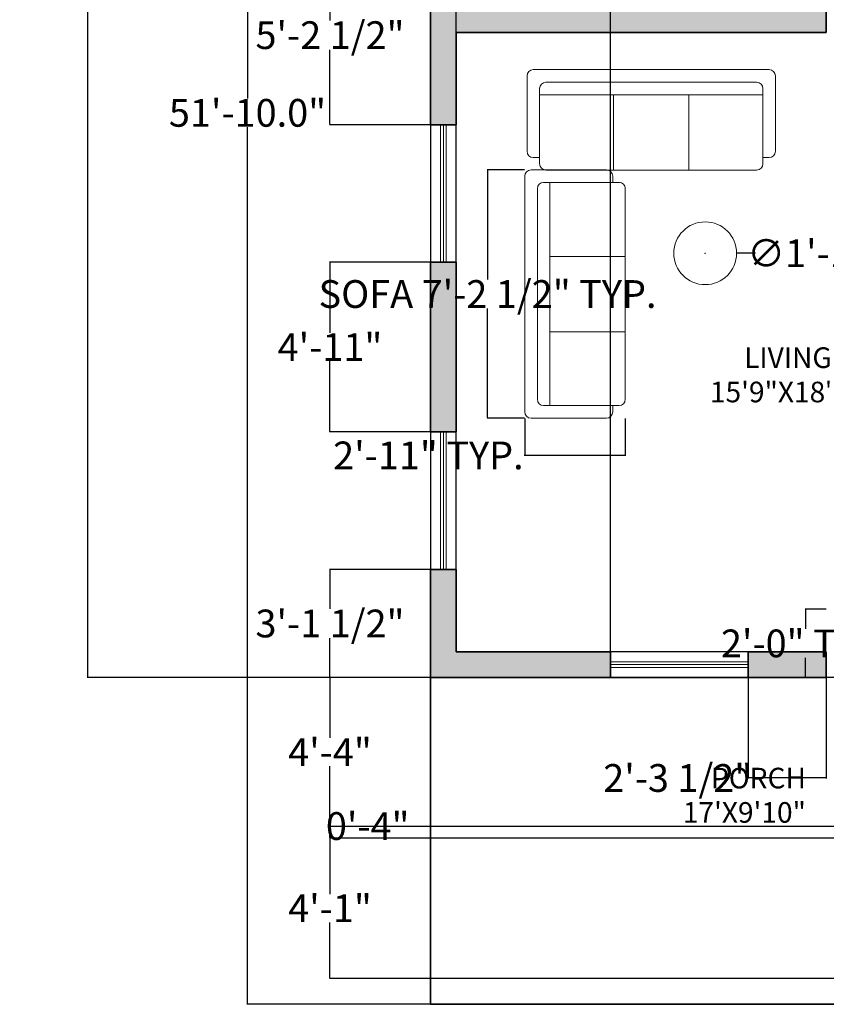
# Model space of a CAD drawing. Units: inches. Extents: x 2103 to 2702, y 2405 to 3142.
# Tile 1 of 7: x 2103 to 2384, y 2447 to 2790. Entities that reach past the tile are written whole.
import ezdxf

# ---------------------------------------------------------------- set-up
doc = ezdxf.new("R2010")
doc.units = ezdxf.units.IN
doc.linetypes.add('0', pattern=[0])
for name, color, linetype, lineweight in [('00 FURNITURE', 15, 'Continuous', 15), ('A-ANNO-DIMS', 2, 'Continuous', 18), ('A-AREA-IDEN', 7, 'Continuous', 18), ('A-WALL-PATT', 8, 'Continuous', 9), ('WALL', 7, 'Continuous', 35), ('WINDOW', 160, '0', 5), ('windows', 4, 'Continuous', 18)]:
    doc.layers.add(name, color=color, linetype=linetype, lineweight=lineweight)
doc.layers.add('furniture', color=34, linetype='Continuous')
doc.styles.get("Standard").update_dxf_attribs({"font": 'arial.ttf'})
doc.dimstyles.get("Standard").update_dxf_attribs({"dimtxt": 9.68, "dimasz": 0.18, "dimexe": 0.18, "dimexo": 0.0625, "dimgap": 0.09, "dimtad": 0, "dimtih": 1, "dimtoh": 1, "dimdec": 1, "dimzin": 0, "dimdsep": 46, "dimlunit": 3, "dimtxsty": 'Standard', "dimcen": 0.09, "dimadec": 0, "dimazin": 0, "dimtfac": 1, "dimtdec": 1, "dimtofl": 0, "dimtmove": 0, "dimatfit": 3, "dimfxl": 1, "dimtolj": 1, "dimtzin": 0, "dimarcsym": 0})

# ---------------------------------------------------------------- blocks, each defined once
blk = doc.blocks.new('window')
at = {"layer": 'furniture'}
for p, q in [((1745.13, 2764.08), (1745.13, 2716.08)), ((1754.13, 2716.08), (1754.13, 2764.08))]:
    blk.add_line(p, q, dxfattribs=at)
at = {"layer": 'WINDOW'}
for p, q in [((1748.63, 2764.08), (1748.63, 2716.08)), ((1749.63, 2764.08), (1749.63, 2716.08)), ((1750.63, 2764.08), (1750.63, 2716.08))]:
    blk.add_line(p, q, dxfattribs=at)
blk = doc.blocks.new('sofa 6')
for p, q in [((-1044.4, 890), (1044.4, 890)), ((-1100, 166.9), (-1100, 834.3)), ((1100, 834.3), (1100, 166.9)), ((-988.8, 55.6), (-988.8, 723.1)), ((-933.1, 778.7), (933.1, 778.7)), ((988.8, 723.1), (988.8, 55.6)), ((-988.8, 667.5), (988.8, 667.5)), ((-333.8, 667.5), (-333.8, 0)), ((333.7, 667.5), (333.7, 0)), ((-988.8, 111.2), (-1044.4, 111.2)), ((1044.4, 111.2), (988.8, 111.2)), ((933.1, 0), (-933.1, 0))]:
    blk.add_line(p, q)
for centre, start, end in [((-1044.4, 834.3), 90, 180), ((1044.4, 834.3), 0, 90), ((-933.1, 723.1), 90, 180), ((933.1, 723.1), 0, 90), ((-1044.4, 166.9), 180, 270), ((1044.4, 166.9), 270, 0), ((-933.1, 55.6), 180, 270), ((933.1, 55.6), 270, 0)]:
    blk.add_arc(centre, 55.6, start, end)
blk = doc.blocks.new('*D16')
at = {"layer": 'A-ANNO-DIMS', "color": 0, "lineweight": -2, "transparency": 16777216}
for p, q in [((2246.37, 3068.85), (2182.44, 3068.85)), ((2182.62, 3068.67), (2182.62, 2762.88)), ((2182.62, 2447.03), (2182.62, 2752.81)), ((2246.37, 2446.85), (2182.44, 2446.85))]:
    blk.add_line(p, q, dxfattribs=at)
at = {"layer": 'A-ANNO-DIMS', "color": 0, "transparency": 16777216}
for points in [[(2182.59, 3068.67), (2182.65, 3068.67), (2182.62, 3068.85)], [(2182.59, 2447.03), (2182.65, 2447.03), (2182.62, 2446.85)]]:
    blk.add_solid(points, dxfattribs=at)
at = {"layer": 'Defpoints', "color": 0, "transparency": 16777216}
for p in [(2246.43, 3068.85), (2182.62, 2446.85), (2246.43, 2446.85)]:
    blk.add_point(p, dxfattribs=at)
at = {"layer": 'A-ANNO-DIMS', "color": 0, "transparency": 16777216, "insert": (2182.62, 2757.85), "char_height": 9.68, "attachment_point": 5}
blk.add_mtext('\\A1;51\'-10.0"', dxfattribs=at)
blk = doc.blocks.new('*D17')
at = {"layer": 'A-ANNO-DIMS', "color": 0, "lineweight": -2, "transparency": 16777216}
for p, q in [((2246.37, 3068.85), (2126.76, 3068.85)), ((2126.94, 3068.67), (2126.94, 2819.88)), ((2126.94, 2561.03), (2126.94, 2809.81)), ((2246.37, 2560.85), (2126.76, 2560.85))]:
    blk.add_line(p, q, dxfattribs=at)
at = {"layer": 'A-ANNO-DIMS', "color": 0, "transparency": 16777216}
for points in [[(2126.91, 3068.67), (2126.97, 3068.67), (2126.94, 3068.85)], [(2126.91, 2561.03), (2126.97, 2561.03), (2126.94, 2560.85)]]:
    blk.add_solid(points, dxfattribs=at)
at = {"layer": 'Defpoints', "color": 0, "transparency": 16777216}
for p in [(2246.43, 3068.85), (2126.94, 2560.85), (2246.43, 2560.85)]:
    blk.add_point(p, dxfattribs=at)
at = {"layer": 'A-ANNO-DIMS', "color": 0, "transparency": 16777216, "insert": (2126.94, 2814.85), "char_height": 9.68, "attachment_point": 5}
blk.add_mtext('\\A1;42\'-4.0"', dxfattribs=at)
blk = doc.blocks.new('*D27')
at = {"layer": 'A-ANNO-DIMS', "color": 0, "lineweight": -2, "transparency": 16777216}
for p, q in [((2384.37, 2584.67), (2377.05, 2584.67)), ((2377.23, 2584.49), (2377.23, 2577.79)), ((2377.23, 2561.03), (2377.23, 2567.72)), ((2384.37, 2560.85), (2377.05, 2560.85))]:
    blk.add_line(p, q, dxfattribs=at)
at = {"layer": 'A-ANNO-DIMS', "color": 0, "transparency": 16777216}
for points in [[(2377.2, 2584.49), (2377.26, 2584.49), (2377.23, 2584.67)], [(2377.2, 2561.03), (2377.26, 2561.03), (2377.23, 2560.85)]]:
    blk.add_solid(points, dxfattribs=at)
at = {"layer": 'Defpoints', "color": 0, "transparency": 16777216}
for p in [(2384.43, 2584.67), (2377.23, 2560.85), (2384.43, 2560.85)]:
    blk.add_point(p, dxfattribs=at)
at = {"layer": 'A-ANNO-DIMS', "color": 0, "transparency": 16777216, "insert": (2377.23, 2572.76), "char_height": 9.68, "attachment_point": 5}
blk.add_mtext('\\A1;2\'-0" TYP.', dxfattribs=at)
blk = doc.blocks.new('*D30')
at = {"layer": 'A-ANNO-DIMS', "color": 0, "lineweight": -2, "transparency": 16777216}
for p, q in [((2279.24, 2737.95), (2266.13, 2737.95)), ((2266.31, 2737.77), (2266.31, 2699.74)), ((2266.31, 2651.51), (2266.31, 2689.54)), ((2279.24, 2651.33), (2266.13, 2651.33))]:
    blk.add_line(p, q, dxfattribs=at)
at = {"layer": 'A-ANNO-DIMS', "color": 0, "transparency": 16777216}
for points in [[(2266.28, 2737.77), (2266.34, 2737.77), (2266.31, 2737.95)], [(2266.28, 2651.51), (2266.34, 2651.51), (2266.31, 2651.33)]]:
    blk.add_solid(points, dxfattribs=at)
at = {"layer": 'Defpoints', "color": 0, "transparency": 16777216}
for p in [(2266.31, 2737.95), (2279.31, 2737.95), (2279.31, 2651.33)]:
    blk.add_point(p, dxfattribs=at)
at = {"layer": 'A-ANNO-DIMS', "color": 0, "transparency": 16777216, "insert": (2266.31, 2694.64), "char_height": 9.68, "attachment_point": 5}
blk.add_mtext('\\A1;SOFA 7\'-2 1/2" TYP.', dxfattribs=at)
blk = doc.blocks.new('*D31')
at = {"layer": 'A-ANNO-DIMS', "color": 0, "lineweight": -2, "transparency": 16777216}
for p, q in [((2279.31, 2651.27), (2279.31, 2638.16)), ((2314.34, 2651.27), (2314.34, 2638.16)), ((2279.31, 2638.34), (2279.13, 2638.34)), ((2314.16, 2638.34), (2279.49, 2638.34))]:
    blk.add_line(p, q, dxfattribs=at)
at = {"layer": 'A-ANNO-DIMS', "color": 0, "transparency": 16777216}
for points in [[(2279.49, 2638.37), (2279.49, 2638.31), (2279.31, 2638.34)], [(2314.16, 2638.37), (2314.16, 2638.31), (2314.34, 2638.34)]]:
    blk.add_solid(points, dxfattribs=at)
at = {"layer": 'Defpoints', "color": 0, "transparency": 16777216}
for p in [(2279.31, 2651.33), (2314.34, 2651.33), (2279.31, 2638.34)]:
    blk.add_point(p, dxfattribs=at)
at = {"layer": 'A-ANNO-DIMS', "color": 0, "transparency": 16777216, "insert": (2245.69, 2638.34), "char_height": 9.68, "attachment_point": 5}
blk.add_mtext('\\A1;2\'-11" TYP.', dxfattribs=at)
blk = doc.blocks.new('*D42')
at = {"layer": 'A-ANNO-DIMS', "color": 0, "lineweight": -2, "transparency": 16777216}
for p, q in [((2471.37, 2504.85), (2211.2, 2504.85)), ((2211.38, 2504.67), (2211.38, 2485.3)), ((2211.38, 2456.03), (2211.38, 2475.4)), ((2471.37, 2455.85), (2211.2, 2455.85))]:
    blk.add_line(p, q, dxfattribs=at)
at = {"layer": 'A-ANNO-DIMS', "color": 0, "transparency": 16777216}
for points in [[(2211.35, 2504.67), (2211.41, 2504.67), (2211.38, 2504.85)], [(2211.35, 2456.03), (2211.41, 2456.03), (2211.38, 2455.85)]]:
    blk.add_solid(points, dxfattribs=at)
at = {"layer": 'Defpoints', "color": 0, "transparency": 16777216}
for p in [(2211.38, 2504.85), (2471.43, 2504.85), (2471.43, 2455.85)]:
    blk.add_point(p, dxfattribs=at)
at = {"layer": 'A-ANNO-DIMS', "color": 0, "transparency": 16777216, "insert": (2211.38, 2480.35), "char_height": 9.68, "attachment_point": 5}
blk.add_mtext('\\A1;4\'-1"', dxfattribs=at)
blk = doc.blocks.new('*D43')
at = {"layer": 'A-ANNO-DIMS', "color": 0, "lineweight": -2, "transparency": 16777216}
for p, q in [((2471.367635, 2560.845674), (2211.200134, 2560.845674)), ((2211.380134, 2560.665674), (2211.380134, 2539.775674)), ((2211.380134, 2509.025674), (2211.380134, 2529.915674)), ((2471.367635, 2508.845674), (2211.200134, 2508.845674))]:
    blk.add_line(p, q, dxfattribs=at)
at = {"layer": 'A-ANNO-DIMS', "color": 0, "transparency": 16777216}
for points in [[(2211.350134, 2560.665674), (2211.410134, 2560.665674), (2211.380134, 2560.845674)], [(2211.350134, 2509.025674), (2211.410134, 2509.025674), (2211.380134, 2508.845674)]]:
    blk.add_solid(points, dxfattribs=at)
at = {"layer": 'Defpoints', "color": 0, "transparency": 16777216}
for p in [(2211.380134, 2560.845674), (2471.430135, 2560.845674), (2471.430135, 2508.845674)]:
    blk.add_point(p, dxfattribs=at)
at = {"layer": 'A-ANNO-DIMS', "color": 0, "transparency": 16777216, "insert": (2211.380134, 2534.845674), "char_height": 9.68, "attachment_point": 5}
blk.add_mtext('\\A1;4\'-4"', dxfattribs=at)
blk = doc.blocks.new('*D47')
at = {"layer": 'A-ANNO-DIMS', "color": 0, "lineweight": -2, "transparency": 16777216}
for p, q in [((2471.37, 2508.85), (2211.2, 2508.85)), ((2211.38, 2508.85), (2211.38, 2509.03)), ((2211.38, 2509.03), (2211.56, 2509.03)), ((2211.38, 2505.03), (2211.38, 2508.67)), ((2471.37, 2504.85), (2211.2, 2504.85))]:
    blk.add_line(p, q, dxfattribs=at)
at = {"layer": 'A-ANNO-DIMS', "color": 0, "transparency": 16777216}
for points in [[(2211.35, 2508.67), (2211.41, 2508.67), (2211.38, 2508.85)], [(2211.35, 2505.03), (2211.41, 2505.03), (2211.38, 2504.85)]]:
    blk.add_solid(points, dxfattribs=at)
at = {"layer": 'Defpoints', "color": 0, "transparency": 16777216}
for p in [(2211.38, 2508.85), (2471.43, 2508.85), (2471.43, 2504.85)]:
    blk.add_point(p, dxfattribs=at)
at = {"layer": 'A-ANNO-DIMS', "color": 0, "transparency": 16777216, "insert": (2224.52, 2509.03), "char_height": 9.68, "attachment_point": 5}
blk.add_mtext('\\A1;0\'-4"', dxfattribs=at)
blk = doc.blocks.new('*D48')
at = {"layer": 'A-ANNO-DIMS', "color": 0, "lineweight": -2, "transparency": 16777216}
for p, q in [((2255.43, 2569.91), (2255.43, 3118.9)), ((2255.61, 3118.72), (2257.85, 3118.72)), ((2308.95, 3118.72), (2306.71, 3118.72)), ((2309.13, 2569.91), (2309.13, 3118.9))]:
    blk.add_line(p, q, dxfattribs=at)
at = {"layer": 'A-ANNO-DIMS', "color": 0, "transparency": 16777216}
for points in [[(2255.61, 3118.75), (2255.61, 3118.69), (2255.43, 3118.72)], [(2308.95, 3118.75), (2308.95, 3118.69), (2309.13, 3118.72)]]:
    blk.add_solid(points, dxfattribs=at)
at = {"layer": 'Defpoints', "color": 0, "transparency": 16777216}
for p in [(2309.13, 3118.72), (2255.43, 2569.85), (2309.13, 2569.85)]:
    blk.add_point(p, dxfattribs=at)
at = {"layer": 'A-ANNO-DIMS', "color": 0, "transparency": 16777216, "insert": (2282.28, 3118.72), "char_height": 9.68, "attachment_point": 5}
blk.add_mtext('\\A1;4\'-5 1/2"', dxfattribs=at)
blk = doc.blocks.new('*D49')
at = {"layer": 'A-ANNO-DIMS', "color": 0, "lineweight": -2, "transparency": 16777216}
for p, q in [((2357.13, 2560.78), (2357.13, 2525.62)), ((2384.43, 2560.78), (2384.43, 2525.62)), ((2357.13, 2525.8), (2356.95, 2525.8)), ((2384.25, 2525.8), (2357.31, 2525.8))]:
    blk.add_line(p, q, dxfattribs=at)
at = {"layer": 'A-ANNO-DIMS', "color": 0, "transparency": 16777216}
for points in [[(2357.31, 2525.83), (2357.31, 2525.77), (2357.13, 2525.8)], [(2384.25, 2525.83), (2384.25, 2525.77), (2384.43, 2525.8)]]:
    blk.add_solid(points, dxfattribs=at)
at = {"layer": 'Defpoints', "color": 0, "transparency": 16777216}
for p in [(2357.13, 2560.85), (2384.43, 2560.85), (2357.13, 2525.8)]:
    blk.add_point(p, dxfattribs=at)
at = {"layer": 'A-ANNO-DIMS', "color": 0, "transparency": 16777216, "insert": (2332.63, 2525.8), "char_height": 9.68, "attachment_point": 5}
blk.add_mtext('\\A1;2\'-3 1/2"', dxfattribs=at)
blk = doc.blocks.new('*D51')
at = {"layer": 'A-ANNO-DIMS', "color": 0, "lineweight": -2, "transparency": 16777216}
for p, q in [((2246.37, 2598.55), (2211.2, 2598.55)), ((2211.38, 2598.37), (2211.38, 2584.8)), ((2211.38, 2561.03), (2211.38, 2574.6)), ((2246.37, 2560.85), (2211.2, 2560.85))]:
    blk.add_line(p, q, dxfattribs=at)
at = {"layer": 'A-ANNO-DIMS', "color": 0, "transparency": 16777216}
for points in [[(2211.35, 2598.37), (2211.41, 2598.37), (2211.38, 2598.55)], [(2211.35, 2561.03), (2211.41, 2561.03), (2211.38, 2560.85)]]:
    blk.add_solid(points, dxfattribs=at)
at = {"layer": 'Defpoints', "color": 0, "transparency": 16777216}
for p in [(2211.38, 2598.55), (2246.43, 2598.55), (2246.43, 2560.85)]:
    blk.add_point(p, dxfattribs=at)
at = {"layer": 'A-ANNO-DIMS', "color": 0, "transparency": 16777216, "insert": (2211.38, 2579.7), "char_height": 9.68, "attachment_point": 5}
blk.add_mtext('\\A1;3\'-1 1/2"', dxfattribs=at)
blk = doc.blocks.new('*D52')
at = {"layer": 'A-ANNO-DIMS', "color": 0, "lineweight": -2, "transparency": 16777216}
for p, q in [((2246.37, 2705.7), (2211.2, 2705.7)), ((2211.38, 2705.52), (2211.38, 2681.08)), ((2211.38, 2646.73), (2211.38, 2671.18)), ((2246.37, 2646.55), (2211.2, 2646.55))]:
    blk.add_line(p, q, dxfattribs=at)
at = {"layer": 'A-ANNO-DIMS', "color": 0, "transparency": 16777216}
for points in [[(2211.35, 2705.52), (2211.41, 2705.52), (2211.38, 2705.7)], [(2211.35, 2646.73), (2211.41, 2646.73), (2211.38, 2646.55)]]:
    blk.add_solid(points, dxfattribs=at)
at = {"layer": 'Defpoints', "color": 0, "transparency": 16777216}
for p in [(2211.38, 2705.7), (2246.43, 2705.7), (2246.43, 2646.55)]:
    blk.add_point(p, dxfattribs=at)
at = {"layer": 'A-ANNO-DIMS', "color": 0, "transparency": 16777216, "insert": (2211.38, 2676.13), "char_height": 9.68, "attachment_point": 5}
blk.add_mtext('\\A1;4\'-11"', dxfattribs=at)
blk = doc.blocks.new('*D53')
at = {"layer": 'A-ANNO-DIMS', "color": 0, "lineweight": -2, "transparency": 16777216}
for p, q in [((2246.37, 2816.19), (2211.2, 2816.19)), ((2211.38, 2816.01), (2211.38, 2790.04)), ((2211.38, 2753.88), (2211.38, 2779.85)), ((2246.37, 2753.7), (2211.2, 2753.7))]:
    blk.add_line(p, q, dxfattribs=at)
at = {"layer": 'A-ANNO-DIMS', "color": 0, "transparency": 16777216}
for points in [[(2211.35, 2816.01), (2211.41, 2816.01), (2211.38, 2816.19)], [(2211.35, 2753.88), (2211.41, 2753.88), (2211.38, 2753.7)]]:
    blk.add_solid(points, dxfattribs=at)
at = {"layer": 'Defpoints', "color": 0, "transparency": 16777216}
for p in [(2211.38, 2816.19), (2246.43, 2816.19), (2246.43, 2753.7)]:
    blk.add_point(p, dxfattribs=at)
at = {"layer": 'A-ANNO-DIMS', "color": 0, "transparency": 16777216, "insert": (2211.38, 2784.95), "char_height": 9.68, "attachment_point": 5}
blk.add_mtext('\\A1;5\'-2 1/2"', dxfattribs=at)
blk = doc.blocks.new('*D78')
at = {"layer": 'A-ANNO-DIMS', "color": 0, "lineweight": -2, "transparency": 16777216}
for p, q in [((2342.12, 2708.86), (2342.3, 2708.86)), ((2342.21, 2708.77), (2342.21, 2708.95)), ((2359.73, 2708.87), (2353.34, 2708.86))]:
    blk.add_line(p, q, dxfattribs=at)
at = {"layer": 'A-ANNO-DIMS', "color": 0, "transparency": 16777216}
blk.add_solid([(2353.34, 2708.9), (2353.34, 2708.84), (2353.16, 2708.86)], dxfattribs=at)
at = {"layer": 'Defpoints', "color": 0, "transparency": 16777216}
for p in [(2331.26, 2708.86), (2353.16, 2708.86)]:
    blk.add_point(p, dxfattribs=at)
at = {"layer": 'A-ANNO-DIMS', "color": 0, "transparency": 16777216, "insert": (2381.71, 2708.87), "char_height": 9.68, "attachment_point": 5}
blk.add_mtext('\\A1;∅1\'-10"', dxfattribs=at)

msp = doc.modelspace()

# ---------------------------------------------------------------- hatches: boundary and pattern name
at = {"layer": 'A-WALL-PATT'}
h = msp.add_hatch(color=256, dxfattribs=at)
h.dxf.hatch_style = 1
h.paths.add_polyline_path([(2342.43, 2911.85), (2342.43, 2915.85), (2255.43, 2915.85), (2255.43, 2976.23), (2246.43, 2976.23), (2246.43, 2840.19), (2255.43, 2840.19), (2255.43, 2854.85), (2315.43, 2854.85), (2315.43, 2845.85), (2319.43, 2845.85), (2319.43, 2858.85), (2255.43, 2858.85), (2255.43, 2906.85), (2342.43, 2906.85)])
h.paths.add_polyline_path([(2384.43, 2794.85), (2319.43, 2794.85), (2319.43, 2815.85), (2315.43, 2815.85), (2315.43, 2794.85), (2255.43, 2794.85), (2255.43, 2816.19), (2246.43, 2816.19), (2246.43, 2753.7), (2255.43, 2753.7), (2255.43, 2785.85), (2384.43, 2785.85)])
h.paths.add_polyline_path([(2606.43, 2963.85), (2597.43, 2963.85), (2597.43, 2951.85), (2537.43, 2951.85), (2537.43, 2957.85), (2533.43, 2957.85), (2533.43, 2951.85), (2469.43, 2951.85), (2444.43, 2951.85), (2444.43, 2842.85), (2449.43, 2842.85), (2453.43, 2842.85), (2453.43, 2942.85), (2597.43, 2942.85), (2597.43, 2904.89), (2606.43, 2904.89)])
h.paths.add_polyline_path([(2606.43, 3019.85), (2597.43, 3019.85), (2597.43, 3003.85), (2537.43, 3003.85), (2537.43, 3015.85), (2533.43, 3015.85), (2533.43, 2987.85), (2537.43, 2987.85), (2537.43, 2999.85), (2597.43, 2999.85), (2597.43, 2987.85), (2606.43, 2987.85)])
h.paths.add_polyline_path([(2606.43, 2856.89), (2597.43, 2856.89), (2597.43, 2774.85), (2552.43, 2774.85), (2552.43, 2765.85), (2597.43, 2765.85), (2597.43, 2749.52), (2606.43, 2749.52)])
h.paths.add_polyline_path([(2522.43, 2774.85), (2453.43, 2774.85), (2453.43, 2806.85), (2444.43, 2806.85), (2444.43, 2794.85), (2432.43, 2794.85), (2432.43, 2785.85), (2444.43, 2785.85), (2444.43, 2765.85), (2453.43, 2765.85), (2509.43, 2765.85), (2509.43, 2705.85), (2498.43, 2705.85), (2498.43, 2701.85), (2597.43, 2701.85), (2597.43, 2678.29), (2606.43, 2678.29), (2606.43, 2725.52), (2597.43, 2725.52), (2597.43, 2705.85), (2513.43, 2705.85), (2513.43, 2765.85), (2522.43, 2765.85)])
h.paths.add_polyline_path([(2255.43, 2705.7), (2246.43, 2705.7), (2246.43, 2646.55), (2255.43, 2646.55)])
h.paths.add_polyline_path([(2255.43, 2598.55), (2246.43, 2598.55), (2246.43, 2560.85), (2309.13, 2560.85), (2309.13, 2569.85), (2309.13, 2569.85), (2255.43, 2569.85)])
h.paths.add_polyline_path([(2495.43, 2569.85), (2495.43, 2569.85), (2453.43, 2569.85), (2453.43, 2701.85), (2462.43, 2701.85), (2462.43, 2705.85), (2444.43, 2705.85), (2444.43, 2569.85), (2432.43, 2569.85), (2432.43, 2564.45), (2432.43, 2564.45), (2432.43, 2560.85), (2495.43, 2560.85)])
h.paths.add_polyline_path([(2384.43, 2569.85), (2357.13, 2569.85), (2357.13, 2560.85), (2384.43, 2560.85)])
h.paths.add_polyline_path([(2606.43, 2630.29), (2597.43, 2630.29), (2597.43, 2569.85), (2543.43, 2569.85), (2543.43, 2560.85), (2597.43, 2560.85), (2597.43, 2455.85), (2450.43, 2455.85), (2450.43, 2446.85), (2606.43, 2446.85)])

# ---------------------------------------------------------------- linework, layer by layer
at = {"layer": '00 FURNITURE'}
msp.add_circle((2342.21, 2708.86), 10.95, dxfattribs=at)
at = {"layer": 'WALL'}
for p, q in [((2246.43, 2816.19), (2246.43, 2753.7)), ((2384.43, 2794.85), (2384.43, 2785.85)), ((2255.43, 2785.85), (2384.43, 2785.85)), ((2255.43, 2785.85), (2255.43, 2753.7)), ((2246.43, 2753.7), (2255.43, 2753.7)), ((2246.43, 2705.7), (2255.43, 2705.7)), ((2246.43, 2705.7), (2246.43, 2646.55)), ((2255.43, 2705.7), (2255.43, 2646.55)), ((2255.43, 2646.55), (2246.43, 2646.55)), ((2255.43, 2598.55), (2246.43, 2598.55)), ((2246.43, 2598.55), (2246.43, 2446.85)), ((2255.43, 2598.55), (2255.43, 2569.85)), ((2255.43, 2569.85), (2309.13, 2569.85)), ((2309.13, 2569.85), (2309.13, 2560.85)), ((2357.13, 2569.85), (2357.13, 2560.85)), ((2357.13, 2569.85), (2384.43, 2569.85)), ((2384.43, 2569.85), (2384.43, 2560.85)), ((2246.43, 2560.85), (2309.13, 2560.85)), ((2357.13, 2560.85), (2384.43, 2560.85)), ((2606.43, 2446.85), (2246.43, 2446.85))]:
    msp.add_line(p, q, dxfattribs=at)

# ---------------------------------------------------------------- block references
at = {"layer": '00 FURNITURE', "xscale": 0.0393700787401575, "yscale": 0.0393700787401575, "zscale": 0.0393700787401575}
msp.add_blockref('sofa 6', (2323.39, 2737.88), dxfattribs=at)
at = {"layer": '00 FURNITURE', "xscale": 0.0393700787401575, "yscale": 0.0393700787401575, "zscale": 0.0393700787401575, "rotation": 90.00000000000047}
msp.add_blockref('sofa 6', (2314.34, 2694.64), dxfattribs=at)
at = {"layer": 'windows'}
for p, rotation in [((4000.56, 5469.78), 180), ((4000.56, 5362.63), 180), ((-406.95, 4314.97), 270)]:
    msp.add_blockref('window', p, dxfattribs=dict(at, rotation=rotation))

# ---------------------------------------------------------------- texts
at = {"layer": 'A-AREA-IDEN', "attachment_point": 3}
for s, insert, char_height in [('LIVING \\P15\'9"X18{\\H0.83478x;\'}', (2386.33, 2676.03), 7.1875), ('PORCH\\P17\'X9\'10"', (2377.33, 2529.36), 7.188)]:
    msp.add_mtext_dynamic_manual_height_columns(s, width=41.3807, gutter_width=12.5, heights=[0], dxfattribs=dict(at, insert=insert, char_height=char_height))

# ---------------------------------------------------------------- dimensions: what is measured, and where the dimension line sits
at = {"layer": 'A-ANNO-DIMS'}
dim = msp.add_linear_dim(base=(2309.13, 3118.72), p1=(2255.43, 2569.85), p2=(2309.13, 2569.85), dimstyle='Standard', override={"dimdec": 1, "dimlfac": 1, "dimrnd": 0, "dimzin": 1, "dimdsep": 46, "dimlunit": 4, "dimfrac": 2}, dxfattribs=at)
dim.commit()
dim.dimension.update_dxf_attribs({"geometry": '*D48', "text_midpoint": (2282.28, 3118.72)})
for base, p1, p2, angle, override, picture, middle in [((2126.94, 2560.85), (2246.43, 3068.85), (2246.43, 2560.85), 90, {"dimclrd": 0, "dimclre": 0, "dimclrt": 0}, '*D17', (2126.94, 2814.85)), ((2182.62, 2446.85), (2246.43, 3068.85), (2246.43, 2446.85), 90, {"dimclrd": 0, "dimclre": 0, "dimclrt": 0}, '*D16', (2182.62, 2757.85)), ((2211.38, 2816.19), (2246.43, 2753.7), (2246.43, 2816.19), 90, {"dimdec": 1, "dimlfac": 1, "dimrnd": 0, "dimzin": 1, "dimdsep": 46, "dimlunit": 4, "dimfrac": 2}, '*D53', (2211.38, 2784.95)), ((2211.3801, 2705.7033), (2246.4301, 2646.5484), (2246.4301, 2705.7033), 90, {"dimdec": 1, "dimlfac": 1, "dimrnd": 0, "dimzin": 1, "dimdsep": 46, "dimlunit": 4, "dimfrac": 2}, '*D52', (2211.3801, 2676.1259)), ((2211.38, 2598.55), (2246.43, 2560.85), (2246.43, 2598.55), 90, {"dimdec": 1, "dimlfac": 1, "dimrnd": 0, "dimzin": 1, "dimdsep": 46, "dimlunit": 4, "dimfrac": 2}, '*D51', (2211.38, 2579.7)), ((2211.38, 2560.85), (2471.43, 2508.85), (2471.43, 2560.85), 90, {"dimdec": 1, "dimlfac": 1, "dimrnd": 0, "dimzin": 1, "dimdsep": 46, "dimlunit": 4, "dimfrac": 2}, '*D43', (2211.38, 2534.85)), ((2357.13, 2525.8), (2384.43, 2560.85), (2357.13, 2560.85), 180, {"dimdec": 1, "dimlfac": 1, "dimrnd": 0, "dimzin": 1, "dimdsep": 46, "dimlunit": 4, "dimfrac": 2}, '*D49', (2332.63, 2525.8)), ((2211.38, 2508.85), (2471.43, 2504.85), (2471.43, 2508.85), 90, {"dimdec": 1, "dimlfac": 1, "dimrnd": 0, "dimzin": 1, "dimdsep": 46, "dimlunit": 4, "dimfrac": 2}, '*D47', (2224.52, 2509.03)), ((2211.38, 2504.85), (2471.43, 2455.85), (2471.43, 2504.85), 90, {"dimdec": 1, "dimlfac": 1, "dimrnd": 0, "dimzin": 1, "dimdsep": 46, "dimlunit": 4, "dimfrac": 2}, '*D42', (2211.38, 2480.35))]:
    dim = msp.add_linear_dim(base=base, p1=p1, p2=p2, angle=angle, dimstyle='Standard', override=override, dxfattribs=at)
    dim.commit()
    dim.dimension.update_dxf_attribs({"geometry": picture, "text_midpoint": middle})
for base, p1, p2, angle, text, picture, middle in [((2266.31, 2737.95), (2279.31, 2651.33), (2279.31, 2737.95), 90, 'SOFA <> TYP.', '*D30', (2266.31, 2694.64)), ((2279.31, 2638.34), (2314.34, 2651.33), (2279.31, 2651.33), 180, '<> TYP.', '*D31', (2245.69, 2638.34)), ((2377.23, 2560.85), (2384.43, 2584.67), (2384.43, 2560.85), 270, '<> TYP.', '*D27', (2377.23, 2572.76))]:
    dim = msp.add_linear_dim(base=base, p1=p1, p2=p2, angle=angle, text=text, dimstyle='Standard', override={"dimdec": 1, "dimlfac": 1, "dimrnd": 0, "dimzin": 1, "dimdsep": 46, "dimlunit": 4, "dimfrac": 2}, dxfattribs=at)
    dim.commit()
    dim.dimension.update_dxf_attribs({"geometry": picture, "text_midpoint": middle})
dim = msp.add_diameter_dim_2p(p1=(2331.26, 2708.86), p2=(2353.16, 2708.86), dimstyle='Standard', override={"dimdec": 1, "dimlfac": 1, "dimrnd": 0, "dimzin": 1, "dimdsep": 46, "dimlunit": 4, "dimfrac": 2}, dxfattribs=at)
dim.commit()
dim.dimension.update_dxf_attribs({"geometry": '*D78', "text_midpoint": (2359.73, 2708.87), "dimtype": 163})

doc.saveas('drawing.dxf')
